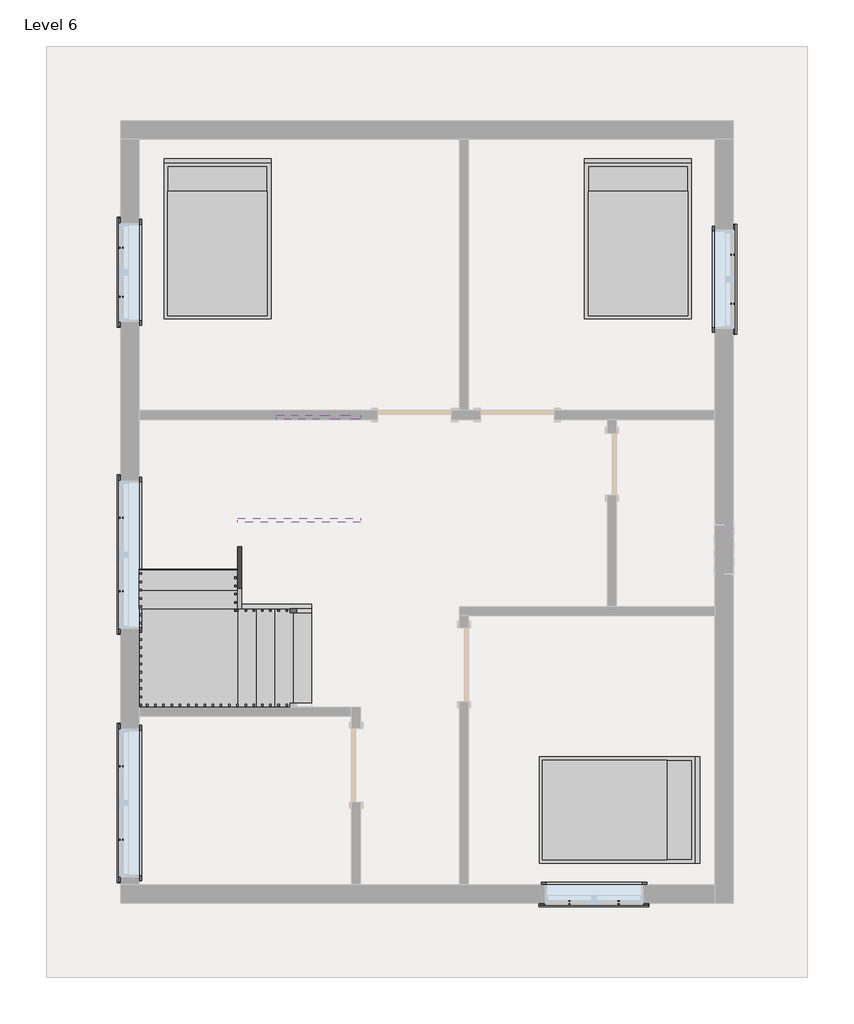
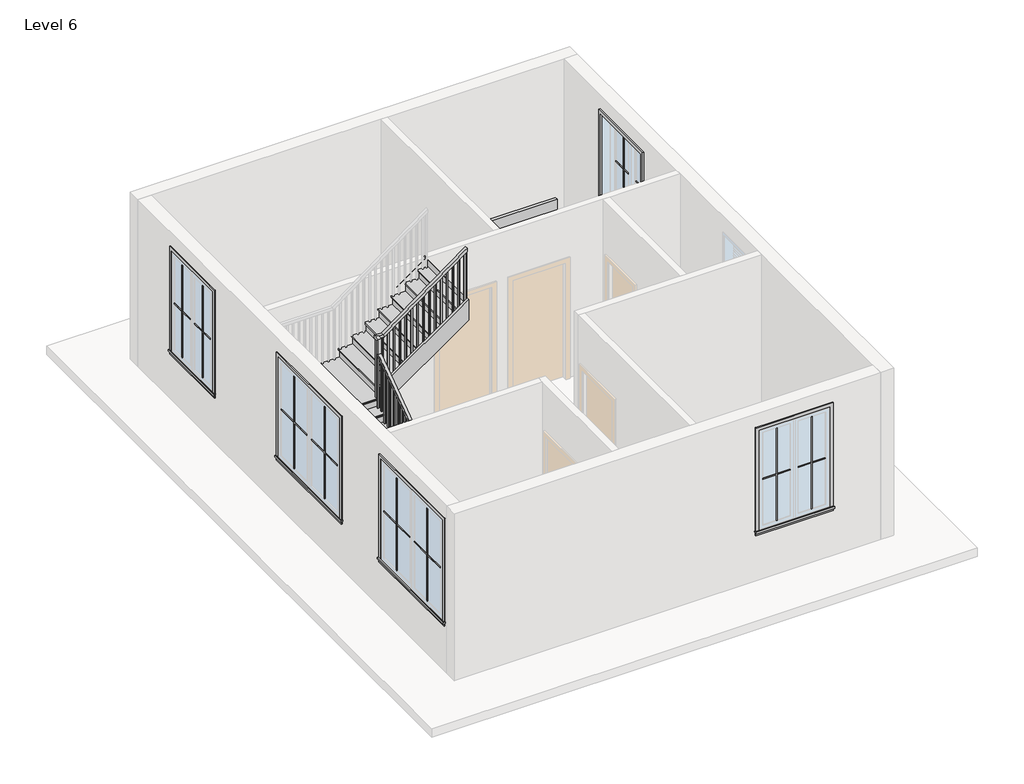
# One storey, part 2 of 2: 20 proxies, 5 members, 3 furniture elements, 1 railing, 1 stair flight.
"""IFC4 building model written with IfcOpenShell, lengths in millimetres."""

from ifc_helpers import new_model, si_unit, frame, origin, place, context, project, spatial, polyline, outline, extrude, faceted_brep, transform, mapped, element, save
from components import muntin_pattern_2x2_muntin_pattern_2x2_0a037076, muntin_pattern_2x2_muntin_pattern_2x2_e6f69628, muntin_pattern_2x2_muntin_pattern_2x2_2b4d9f72, muntin_pattern_2x2_muntin_pattern_2x2_ef995ed3, trim_window_exterior_flat_with_sill_b601e94a, trim_window_exterior_flat_with_sill_b7e4d11c, trim_window_interior_flat_picture_frame_bfefb25c, trim_window_interior_flat_picture_frame_936b8d2a, bed_17739_bed_17739_15c61121, stair_flight_8c9b7ea6

model = new_model("IFC4")

# Units and contexts
model_context = context("Model", 3, world=origin())
ifc_project = project(units=[si_unit("LENGTHUNIT", "METRE", prefix="MILLI")], contexts=[model_context])

# Site, building, storey
site = spatial("IfcSite", under=ifc_project)
building = spatial("IfcBuilding", under=site)
storey = spatial("IfcBuildingStorey", under=building, Name="Level 6", Elevation=15849.6)

# Proxies
placement = place(None, origin())
muntin_pattern_2x2_muntin_pattern_2x2_shape = muntin_pattern_2x2_muntin_pattern_2x2_0a037076(model_context)
element("IfcBuildingElementProxy", 1, Name="Muntin Pattern_2x2 : Muntin Pattern_2x2", ObjectType="Muntin Pattern_2x2 : Muntin Pattern_2x2", at=placement, inside=storey, context=model_context, shape_type="MappedRepresentation", body=[
    mapped(muntin_pattern_2x2_muntin_pattern_2x2_shape, transform((-5035.7855391, -4380.9248761, 16833.85), x_axis=(0.0, 1.0, 0.0), y_axis=(-1.0, 0.0, 0.0), z_axis=(0.0, 0.0, 1.0))),
])
element("IfcBuildingElementProxy", 2, Name="Muntin Pattern_2x2 : Muntin Pattern_2x2", ObjectType="Muntin Pattern_2x2 : Muntin Pattern_2x2", at=placement, inside=storey, context=model_context, shape_type="MappedRepresentation", body=[
    mapped(muntin_pattern_2x2_muntin_pattern_2x2_shape, transform((-5035.7855391, -1310.6998761, 16833.85), x_axis=(0.0, 1.0, 0.0), y_axis=(-1.0, 0.0, 0.0), z_axis=(0.0, 0.0, 1.0))),
])
muntin_pattern_2x2_muntin_pattern_2x2_2_shape = muntin_pattern_2x2_muntin_pattern_2x2_e6f69628(model_context)
element("IfcBuildingElementProxy", 3, Name="Muntin Pattern_2x2 : Muntin Pattern_2x2", ObjectType="Muntin Pattern_2x2 : Muntin Pattern_2x2", at=placement, inside=storey, context=model_context, shape_type="MappedRepresentation", body=[
    mapped(muntin_pattern_2x2_muntin_pattern_2x2_2_shape, transform((-5035.7855391, -3469.6998761, 16833.85), x_axis=(0.0, -1.0, 0.0), y_axis=(1.0, 0.0, 0.0), z_axis=(0.0, 0.0, 1.0))),
])
element("IfcBuildingElementProxy", 4, Name="Muntin Pattern_2x2 : Muntin Pattern_2x2", ObjectType="Muntin Pattern_2x2 : Muntin Pattern_2x2", at=placement, inside=storey, context=model_context, shape_type="MappedRepresentation", body=[
    mapped(muntin_pattern_2x2_muntin_pattern_2x2_2_shape, transform((-5035.7855391, -399.4748761, 16833.85), x_axis=(0.0, -1.0, 0.0), y_axis=(1.0, 0.0, 0.0), z_axis=(0.0, 0.0, 1.0))),
])
muntin_pattern_2x2_muntin_pattern_2x2_3_shape = muntin_pattern_2x2_muntin_pattern_2x2_2b4d9f72(model_context)
element("IfcBuildingElementProxy", 5, Name="Muntin Pattern_2x2 : Muntin Pattern_2x2", ObjectType="Muntin Pattern_2x2 : Muntin Pattern_2x2", at=placement, inside=storey, context=model_context, shape_type="MappedRepresentation", body=[
    mapped(muntin_pattern_2x2_muntin_pattern_2x2_3_shape, transform((1115.7769609, -5157.2123761, 16833.85), x_axis=(-1.0, 0.0, 0.0), y_axis=(0.0, -1.0, 0.0), z_axis=(0.0, 0.0, 1.0))),
])
element("IfcBuildingElementProxy", 6, Name="Muntin Pattern_2x2 : Muntin Pattern_2x2", ObjectType="Muntin Pattern_2x2 : Muntin Pattern_2x2", at=placement, inside=storey, context=model_context, shape_type="MappedRepresentation", body=[
    mapped(muntin_pattern_2x2_muntin_pattern_2x2_3_shape, transform((2527.0644609, 2851.7251239, 16833.85), x_axis=(0.0, -1.0, 0.0), y_axis=(1.0, 0.0, 0.0), z_axis=(0.0, 0.0, 1.0))),
])
element("IfcBuildingElementProxy", 7, Name="Muntin Pattern_2x2 : Muntin Pattern_2x2", ObjectType="Muntin Pattern_2x2 : Muntin Pattern_2x2", at=placement, inside=storey, context=model_context, shape_type="MappedRepresentation", body=[
    mapped(muntin_pattern_2x2_muntin_pattern_2x2_3_shape, transform((-5035.7855391, 2331.0251239, 16833.85), x_axis=(0.0, 1.0, 0.0), y_axis=(-1.0, 0.0, 0.0), z_axis=(0.0, 0.0, 1.0))),
])
muntin_pattern_2x2_muntin_pattern_2x2_4_shape = muntin_pattern_2x2_muntin_pattern_2x2_ef995ed3(model_context)
element("IfcBuildingElementProxy", 8, Name="Muntin Pattern_2x2 : Muntin Pattern_2x2", ObjectType="Muntin Pattern_2x2 : Muntin Pattern_2x2", at=placement, inside=storey, context=model_context, shape_type="MappedRepresentation", body=[
    mapped(muntin_pattern_2x2_muntin_pattern_2x2_4_shape, transform((509.3519609, -5157.2123761, 16833.85), x_axis=(1.0, 0.0, 0.0), y_axis=(0.0, 1.0, 0.0), z_axis=(0.0, 0.0, 1.0))),
])
element("IfcBuildingElementProxy", 9, Name="Muntin Pattern_2x2 : Muntin Pattern_2x2", ObjectType="Muntin Pattern_2x2 : Muntin Pattern_2x2", at=placement, inside=storey, context=model_context, shape_type="MappedRepresentation", body=[
    mapped(muntin_pattern_2x2_muntin_pattern_2x2_4_shape, transform((2527.0644609, 2245.3001239, 16833.85), x_axis=(0.0, 1.0, 0.0), y_axis=(-1.0, 0.0, 0.0), z_axis=(0.0, 0.0, 1.0))),
])
element("IfcBuildingElementProxy", 10, Name="Muntin Pattern_2x2 : Muntin Pattern_2x2", ObjectType="Muntin Pattern_2x2 : Muntin Pattern_2x2", at=placement, inside=storey, context=model_context, shape_type="MappedRepresentation", body=[
    mapped(muntin_pattern_2x2_muntin_pattern_2x2_4_shape, transform((-5035.7855391, 2937.4501239, 16833.85), x_axis=(0.0, -1.0, 0.0), y_axis=(1.0, 0.0, 0.0), z_axis=(0.0, 0.0, 1.0))),
])
trim_window_exterior_flat_with_sill_shape = trim_window_exterior_flat_with_sill_b601e94a(model_context)
element("IfcBuildingElementProxy", 11, Name="Trim-Window-Exterior-Flat : with Sill", ObjectType="Trim-Window-Exterior-Flat : with Sill", at=placement, inside=storey, context=model_context, shape_type="MappedRepresentation", body=[
    mapped(trim_window_exterior_flat_with_sill_shape, transform((-5045.3105391, -3925.3123761, 18592.8), x_axis=(0.0, -1.0, 0.0), y_axis=(0.0, 0.0, 1.0), z_axis=(-1.0, 0.0, 0.0))),
])
element("IfcBuildingElementProxy", 12, Name="Trim-Window-Exterior-Flat : with Sill", ObjectType="Trim-Window-Exterior-Flat : with Sill", at=placement, inside=storey, context=model_context, shape_type="MappedRepresentation", body=[
    mapped(trim_window_exterior_flat_with_sill_shape, transform((-5045.3105391, -855.0873761, 18592.8), x_axis=(0.0, -1.0, 0.0), y_axis=(0.0, 0.0, 1.0), z_axis=(-1.0, 0.0, 0.0))),
])
trim_window_exterior_flat_with_sill_2_shape = trim_window_exterior_flat_with_sill_b7e4d11c(model_context)
element("IfcBuildingElementProxy", 13, Name="Trim-Window-Exterior-Flat : with Sill", ObjectType="Trim-Window-Exterior-Flat : with Sill", at=placement, inside=storey, context=model_context, shape_type="MappedRepresentation", body=[
    mapped(trim_window_exterior_flat_with_sill_2_shape, transform((812.5644609, -5166.7373761, 18592.8), x_axis=(1.0, 0.0, 0.0), y_axis=(0.0, 0.0, 1.0), z_axis=(0.0, -1.0, 0.0))),
])
element("IfcBuildingElementProxy", 14, Name="Trim-Window-Exterior-Flat : with Sill", ObjectType="Trim-Window-Exterior-Flat : with Sill", at=placement, inside=storey, context=model_context, shape_type="MappedRepresentation", body=[
    mapped(trim_window_exterior_flat_with_sill_2_shape, transform((2536.5894609, 2548.5126239, 18592.8), x_axis=(0.0, 1.0, 0.0), y_axis=(0.0, 0.0, 1.0), z_axis=(1.0, 0.0, 0.0))),
])
element("IfcBuildingElementProxy", 15, Name="Trim-Window-Exterior-Flat : with Sill", ObjectType="Trim-Window-Exterior-Flat : with Sill", at=placement, inside=storey, context=model_context, shape_type="MappedRepresentation", body=[
    mapped(trim_window_exterior_flat_with_sill_2_shape, transform((-5045.3105391, 2634.2376239, 18592.8), x_axis=(0.0, -1.0, 0.0), y_axis=(0.0, 0.0, 1.0), z_axis=(-1.0, 0.0, 0.0))),
])
trim_window_interior_flat_picture_frame_shape = trim_window_interior_flat_picture_frame_bfefb25c(model_context)
element("IfcBuildingElementProxy", 16, Name="Trim-Window-Interior-Flat : Picture Frame", ObjectType="Trim-Window-Interior-Flat : Picture Frame", at=placement, inside=storey, context=model_context, shape_type="MappedRepresentation", body=[
    mapped(trim_window_interior_flat_picture_frame_shape, transform((-4816.7105391, -3925.3123761, 18592.8), x_axis=(0.0, 1.0, 0.0), y_axis=(0.0, 0.0, 1.0), z_axis=(1.0, 0.0, 0.0))),
])
element("IfcBuildingElementProxy", 17, Name="Trim-Window-Interior-Flat : Picture Frame", ObjectType="Trim-Window-Interior-Flat : Picture Frame", at=placement, inside=storey, context=model_context, shape_type="MappedRepresentation", body=[
    mapped(trim_window_interior_flat_picture_frame_shape, transform((-4816.7105391, -855.0873761, 18592.8), x_axis=(0.0, 1.0, 0.0), y_axis=(0.0, 0.0, 1.0), z_axis=(1.0, 0.0, 0.0))),
])
trim_window_interior_flat_picture_frame_2_shape = trim_window_interior_flat_picture_frame_936b8d2a(model_context)
element("IfcBuildingElementProxy", 18, Name="Trim-Window-Interior-Flat : Picture Frame", ObjectType="Trim-Window-Interior-Flat : Picture Frame", at=placement, inside=storey, context=model_context, shape_type="MappedRepresentation", body=[
    mapped(trim_window_interior_flat_picture_frame_2_shape, transform((812.5644609, -4938.1373761, 18592.8), x_axis=(-1.0, 0.0, 0.0), y_axis=(0.0, 0.0, 1.0), z_axis=(0.0, 1.0, 0.0))),
])
element("IfcBuildingElementProxy", 19, Name="Trim-Window-Interior-Flat : Picture Frame", ObjectType="Trim-Window-Interior-Flat : Picture Frame", at=placement, inside=storey, context=model_context, shape_type="MappedRepresentation", body=[
    mapped(trim_window_interior_flat_picture_frame_2_shape, transform((2307.9894609, 2548.5126239, 18592.8), x_axis=(0.0, -1.0, 0.0), y_axis=(0.0, 0.0, 1.0), z_axis=(-1.0, 0.0, 0.0))),
])
element("IfcBuildingElementProxy", 20, Name="Trim-Window-Interior-Flat : Picture Frame", ObjectType="Trim-Window-Interior-Flat : Picture Frame", at=placement, inside=storey, context=model_context, shape_type="MappedRepresentation", body=[
    mapped(trim_window_interior_flat_picture_frame_2_shape, transform((-4816.7105391, 2634.2376239, 18592.8), x_axis=(0.0, 1.0, 0.0), y_axis=(0.0, 0.0, 1.0), z_axis=(1.0, 0.0, 0.0))),
])

# Furniture
bed_17739_bed_17739_shape = bed_17739_bed_17739_15c61121(model_context)
element("IfcFurniture", 21, ObjectType="Bed_17739 : Bed_17739", at=placement, inside=storey, context=model_context, shape_type="MappedRepresentation", body=[
    mapped(bed_17739_bed_17739_shape, transform((-3845.1605391, 3024.7626239, 15849.6), x_axis=(1.0, 0.0, 0.0), y_axis=(0.0, 1.0, 0.0), z_axis=(0.0, 0.0, 1.0))),
])
element("IfcFurniture", 22, ObjectType="Bed_17739 : Bed_17739", at=placement, inside=storey, context=model_context, shape_type="MappedRepresentation", body=[
    mapped(bed_17739_bed_17739_shape, transform((1355.4894609, 3024.7626239, 15849.6), x_axis=(1.0, 0.0, 0.0), y_axis=(0.0, 1.0, 0.0), z_axis=(0.0, 0.0, 1.0))),
])
element("IfcFurniture", 23, ObjectType="Bed_17739 : Bed_17739", at=placement, inside=storey, context=model_context, shape_type="MappedRepresentation", body=[
    mapped(bed_17739_bed_17739_shape, transform((1101.4894609, -4011.0373761, 15849.6), x_axis=(0.0, -1.0, 0.0), y_axis=(1.0, 0.0, 0.0), z_axis=(0.0, 0.0, 1.0))),
])

# Members
element("IfcMember", 24, ObjectType="Stringer - 2\" Width", at=placement, inside=storey, context=model_context, shape_type="SweptSolid", body=[
    extrude(outline(polyline([(15849.6, -2683.1105391), (16000.1087903, -2683.1105391), (16000.1087903, -3112.2707489), (15849.6, -2897.7957228), (15849.6, -2683.1105391)])), frame((0.0, -2791.8373761, 0.0), z_axis=(0.0, 1.0, 0.0), x_axis=(0.0, 0.0, 1.0)), (0.0, 0.0, 1.0), 50.8),
])
element("IfcMember", 25, ObjectType="Stringer - 2\" Width", at=placement, inside=storey, context=model_context, shape_type="SweptSolid", body=[
    extrude(outline(polyline([(18177.0856495, -2580.7583047), (18533.0489938, -2073.5105391), (18905.4117181, -2073.5105391), (18177.0856495, -3111.3751869), (18177.0856495, -2580.7583047)])), frame((0.0, 814.9626239, 0.0), z_axis=(0.0, 1.0, 0.0), x_axis=(0.0, 0.0, 1.0)), (0.0, 0.0, 1.0), 50.8),
])
element("IfcMember", 26, ObjectType="Stringer - 2\" Width", at=placement, inside=storey, context=model_context, shape_type="SweptSolid", body=[
    extrude(outline(polyline([(15849.6, -2683.1105391), (16071.306455, -2683.1105391), (16677.3415427, -3546.7105391), (16304.9788184, -3546.7105391), (15849.6, -2897.7957228), (15849.6, -2683.1105391)])), frame((0.0, -1521.8373761, 0.0), z_axis=(0.0, 1.0, 0.0), x_axis=(0.0, 0.0, 1.0)), (0.0, 0.0, 1.0), 50.8),
])
element("IfcMember", 27, ObjectType="Stringer - 2\" Width", at=placement, inside=storey, context=model_context, shape_type="SweptSolid", body=[
    extrude(outline(polyline([(-1521.8373761, 16499.9564629), (-1521.8373761, 16875.1327137), (-455.0373761, 17640.7786467), (-455.0373761, 17265.6023959), (-1521.8373761, 16499.9564629)])), frame((-3597.5105391, 0.0, 0.0), z_axis=(1.0, 0.0, 0.0), x_axis=(0.0, 1.0, 0.0)), (0.0, 0.0, 1.0), 50.8),
])
element("IfcMember", 28, ObjectType="Stringer - 2\" Width", at=placement, inside=storey, context=model_context, shape_type="SweptSolid", body=[
    extrude(outline(polyline([(17835.9380339, -3597.5105391), (17463.5753096, -3597.5105391), (18533.0489938, -2073.5105391), (18905.4117181, -2073.5105391), (17835.9380339, -3597.5105391)])), frame((0.0, -455.0373761, 0.0), z_axis=(0.0, 1.0, 0.0), x_axis=(0.0, 0.0, 1.0)), (0.0, 0.0, 1.0), 50.8),
])

# Railing
element("IfcRailing", 29, ObjectType="Handrail - Rectangular", at=placement, inside=storey, context=model_context, shape_type="SolidModel", body=[
    faceted_brep([(-2683.1105391, -1572.6373761, 16924.4210526), (-2683.1105391, -1572.6373761, 16862.3605986), (-2683.1105391, -1521.8373761, 16862.3605986), (-2683.1105391, -1521.8373761, 16924.4210526), (-3521.3105391, -1572.6373761, 17512.6315789), (-3572.1105391, -1572.6373761, 17486.2202477), (-3572.1105391, -1521.8373761, 17486.2202477), (-3521.3105391, -1521.8373761, 17512.6315789), (-3521.3105391, -1572.6373761, 17781.215311), (-3572.1105391, -1572.6373761, 17730.415311), (-3572.1105391, -1521.8373761, 17730.415311), (-3521.3105391, -1521.8373761, 17781.215311), (-3648.3105391, -1572.6373761, 17781.215311), (-3648.3105391, -1572.6373761, 17730.415311), (-3597.5105391, -1521.8373761, 17730.415311), (-3597.5105391, -1521.8373761, 17781.215311), (-3648.3105391, -1445.6373761, 17781.215311), (-3648.3105391, -1429.2944467, 17730.415311), (-3597.5105391, -1429.2944467, 17730.415311), (-3597.5105391, -1445.6373761, 17781.215311), (-3648.3105391, -480.4373761, 18473.9425837), (-3648.3105391, -429.6373761, 18447.8725387), (-3597.5105391, -429.6373761, 18447.8725387), (-3597.5105391, -480.4373761, 18473.9425837), (-3648.3105391, -480.4373761, 18745.2), (-3648.3105391, -429.6373761, 18694.4), (-3597.5105391, -429.6373761, 18694.4), (-3597.5105391, -480.4373761, 18745.2), (-3648.3105391, -353.4373761, 18745.2), (-3648.3105391, -353.4373761, 18694.4), (-3597.5105391, -404.2373761, 18694.4), (-3597.5105391, -404.2373761, 18745.2), (-3521.3105391, -353.4373761, 18745.2), (-3504.6160355, -353.4373761, 18694.4), (-3504.6160355, -404.2373761, 18694.4), (-3521.3105391, -404.2373761, 18745.2), (-2073.5105391, -353.4373761, 19812.0), (-2073.5105391, -404.2373761, 19812.0), (-2073.5105391, -404.2373761, 19748.8987868), (-2073.5105391, -353.4373761, 19748.8987868)], [[[0, 1, 2, 3]], [[1, 0, 4, 5]], [[2, 1, 5, 6]], [[3, 2, 6, 7]], [[0, 3, 7, 4]], [[5, 4, 8, 9]], [[6, 5, 9, 10]], [[7, 6, 10, 11]], [[4, 7, 11, 8]], [[9, 8, 12, 13]], [[10, 9, 13, 14]], [[11, 10, 14, 15]], [[8, 11, 15, 12]], [[13, 12, 16, 17]], [[14, 13, 17, 18]], [[15, 14, 18, 19]], [[12, 15, 19, 16]], [[17, 16, 20, 21]], [[18, 17, 21, 22]], [[19, 18, 22, 23]], [[16, 19, 23, 20]], [[21, 20, 24, 25]], [[22, 21, 25, 26]], [[23, 22, 26, 27]], [[20, 23, 27, 24]], [[25, 24, 28, 29]], [[26, 25, 29, 30]], [[27, 26, 30, 31]], [[24, 27, 31, 28]], [[29, 28, 32, 33]], [[30, 29, 33, 34]], [[31, 30, 34, 35]], [[28, 31, 35, 32]], [[36, 37, 38, 39]], [[33, 32, 36, 39]], [[34, 33, 39, 38]], [[35, 34, 38, 37]], [[32, 35, 37, 36]]]),
    extrude(outline(polyline([(19737.2014184, -2089.3855391), (19723.1645763, -2108.4355391), (18737.1789474, -2108.4355391), (18737.1789474, -2089.3855391), (19737.2014184, -2089.3855391)])), frame((0.0, -388.3623761, 0.0), z_axis=(0.0, 1.0, 0.0), x_axis=(0.0, 0.0, 1.0)), (0.0, 0.0, 1.0), 19.05),
    extrude(outline(polyline([(19662.3382605, -2190.9855391), (19648.3014184, -2210.0355391), (18737.1789474, -2210.0355391), (18737.1789474, -2190.9855391), (19662.3382605, -2190.9855391)])), frame((0.0, -388.3623761, 0.0), z_axis=(0.0, 1.0, 0.0), x_axis=(0.0, 0.0, 1.0)), (0.0, 0.0, 1.0), 19.05),
    extrude(outline(polyline([(19587.4751026, -2292.5855391), (19573.4382605, -2311.6355391), (18576.7578947, -2311.6355391), (18576.7578947, -2292.5855391), (19587.4751026, -2292.5855391)])), frame((0.0, -388.3623761, 0.0), z_axis=(0.0, 1.0, 0.0), x_axis=(0.0, 0.0, 1.0)), (0.0, 0.0, 1.0), 19.05),
    extrude(outline(polyline([(19512.6119447, -2394.1855391), (19498.5751026, -2413.2355391), (18576.7578947, -2413.2355391), (18576.7578947, -2394.1855391), (19512.6119447, -2394.1855391)])), frame((0.0, -388.3623761, 0.0), z_axis=(0.0, 1.0, 0.0), x_axis=(0.0, 0.0, 1.0)), (0.0, 0.0, 1.0), 19.05),
    extrude(outline(polyline([(19437.7487868, -2495.7855391), (19423.7119447, -2514.8355391), (18416.3368421, -2514.8355391), (18416.3368421, -2495.7855391), (19437.7487868, -2495.7855391)])), frame((0.0, -388.3623761, 0.0), z_axis=(0.0, 1.0, 0.0), x_axis=(0.0, 0.0, 1.0)), (0.0, 0.0, 1.0), 19.05),
    extrude(outline(polyline([(19362.8856289, -2597.3855391), (19348.8487868, -2616.4355391), (18416.3368421, -2616.4355391), (18416.3368421, -2597.3855391), (19362.8856289, -2597.3855391)])), frame((0.0, -388.3623761, 0.0), z_axis=(0.0, 1.0, 0.0), x_axis=(0.0, 0.0, 1.0)), (0.0, 0.0, 1.0), 19.05),
    extrude(outline(polyline([(19288.022471, -2698.9855391), (19273.9856289, -2718.0355391), (18255.9157895, -2718.0355391), (18255.9157895, -2698.9855391), (19288.022471, -2698.9855391)])), frame((0.0, -388.3623761, 0.0), z_axis=(0.0, 1.0, 0.0), x_axis=(0.0, 0.0, 1.0)), (0.0, 0.0, 1.0), 19.05),
    extrude(outline(polyline([(19213.1593132, -2800.5855391), (19199.122471, -2819.6355391), (18255.9157895, -2819.6355391), (18255.9157895, -2800.5855391), (19213.1593132, -2800.5855391)])), frame((0.0, -388.3623761, 0.0), z_axis=(0.0, 1.0, 0.0), x_axis=(0.0, 0.0, 1.0)), (0.0, 0.0, 1.0), 19.05),
    extrude(outline(polyline([(19138.2961553, -2902.1855391), (19124.2593132, -2921.2355391), (18255.9157895, -2921.2355391), (18255.9157895, -2902.1855391), (19138.2961553, -2902.1855391)])), frame((0.0, -388.3623761, 0.0), z_axis=(0.0, 1.0, 0.0), x_axis=(0.0, 0.0, 1.0)), (0.0, 0.0, 1.0), 19.05),
    extrude(outline(polyline([(19063.4329974, -3003.7855391), (19049.3961553, -3022.8355391), (18095.4947368, -3022.8355391), (18095.4947368, -3003.7855391), (19063.4329974, -3003.7855391)])), frame((0.0, -388.3623761, 0.0), z_axis=(0.0, 1.0, 0.0), x_axis=(0.0, 0.0, 1.0)), (0.0, 0.0, 1.0), 19.05),
    extrude(outline(polyline([(18988.5698395, -3105.3855391), (18974.5329974, -3124.4355391), (18095.4947368, -3124.4355391), (18095.4947368, -3105.3855391), (18988.5698395, -3105.3855391)])), frame((0.0, -388.3623761, 0.0), z_axis=(0.0, 1.0, 0.0), x_axis=(0.0, 0.0, 1.0)), (0.0, 0.0, 1.0), 19.05),
    extrude(outline(polyline([(18913.7066816, -3206.9855391), (18899.6698395, -3226.0355391), (17935.0736842, -3226.0355391), (17935.0736842, -3206.9855391), (18913.7066816, -3206.9855391)])), frame((0.0, -388.3623761, 0.0), z_axis=(0.0, 1.0, 0.0), x_axis=(0.0, 0.0, 1.0)), (0.0, 0.0, 1.0), 19.05),
    extrude(outline(polyline([(18838.8435237, -3308.5855391), (18824.8066816, -3327.6355391), (17935.0736842, -3327.6355391), (17935.0736842, -3308.5855391), (18838.8435237, -3308.5855391)])), frame((0.0, -388.3623761, 0.0), z_axis=(0.0, 1.0, 0.0), x_axis=(0.0, 0.0, 1.0)), (0.0, 0.0, 1.0), 19.05),
    extrude(outline(polyline([(18763.9803658, -3410.1855391), (18749.9435237, -3429.2355391), (17774.6526316, -3429.2355391), (17774.6526316, -3410.1855391), (18763.9803658, -3410.1855391)])), frame((0.0, -388.3623761, 0.0), z_axis=(0.0, 1.0, 0.0), x_axis=(0.0, 0.0, 1.0)), (0.0, 0.0, 1.0), 19.05),
    extrude(outline(polyline([(18689.1172079, -3511.7855391), (18675.0803658, -3530.8355391), (17774.6526316, -3530.8355391), (17774.6526316, -3511.7855391), (18689.1172079, -3511.7855391)])), frame((0.0, -388.3623761, 0.0), z_axis=(0.0, 1.0, 0.0), x_axis=(0.0, 0.0, 1.0)), (0.0, 0.0, 1.0), 19.05),
    extrude(outline(polyline([(-3613.3855391, -439.1623761), (-3632.4355391, -439.1623761), (-3632.4355391, -420.1123761), (-3613.3855391, -420.1123761), (-3613.3855391, -439.1623761)])), frame((0.0, 0.0, 17453.8105263), z_axis=(0.0, 0.0, 1.0), x_axis=(1.0, 0.0, 0.0)), (0.0, 0.0, 1.0), 1240.5894737),
    extrude(outline(polyline([(-540.7623761, 18368.1177541), (-521.7123761, 18381.7900029), (-521.7123761, 17453.8105263), (-540.7623761, 17453.8105263), (-540.7623761, 18368.1177541)])), frame((-3632.4355391, 0.0, 0.0), z_axis=(1.0, 0.0, 0.0), x_axis=(0.0, 1.0, 0.0)), (0.0, 0.0, 1.0), 19.05),
    extrude(outline(polyline([(-642.3623761, 18295.1990938), (-623.3123761, 18308.8713426), (-623.3123761, 17293.3894737), (-642.3623761, 17293.3894737), (-642.3623761, 18295.1990938)])), frame((-3632.4355391, 0.0, 0.0), z_axis=(1.0, 0.0, 0.0), x_axis=(0.0, 1.0, 0.0)), (0.0, 0.0, 1.0), 19.05),
    extrude(outline(polyline([(-743.9623761, 18222.2804335), (-724.9123761, 18235.9526823), (-724.9123761, 17293.3894737), (-743.9623761, 17293.3894737), (-743.9623761, 18222.2804335)])), frame((-3632.4355391, 0.0, 0.0), z_axis=(1.0, 0.0, 0.0), x_axis=(0.0, 1.0, 0.0)), (0.0, 0.0, 1.0), 19.05),
    extrude(outline(polyline([(-845.5623761, 18149.3617732), (-826.5123761, 18163.034022), (-826.5123761, 17293.3894737), (-845.5623761, 17293.3894737), (-845.5623761, 18149.3617732)])), frame((-3632.4355391, 0.0, 0.0), z_axis=(1.0, 0.0, 0.0), x_axis=(0.0, 1.0, 0.0)), (0.0, 0.0, 1.0), 19.05),
    extrude(outline(polyline([(-947.1623761, 18076.4431129), (-928.1123761, 18090.1153617), (-928.1123761, 17132.9684211), (-947.1623761, 17132.9684211), (-947.1623761, 18076.4431129)])), frame((-3632.4355391, 0.0, 0.0), z_axis=(1.0, 0.0, 0.0), x_axis=(0.0, 1.0, 0.0)), (0.0, 0.0, 1.0), 19.05),
    extrude(outline(polyline([(-1048.7623761, 18003.5244526), (-1029.7123761, 18017.1967014), (-1029.7123761, 17132.9684211), (-1048.7623761, 17132.9684211), (-1048.7623761, 18003.5244526)])), frame((-3632.4355391, 0.0, 0.0), z_axis=(1.0, 0.0, 0.0), x_axis=(0.0, 1.0, 0.0)), (0.0, 0.0, 1.0), 19.05),
    extrude(outline(polyline([(-1150.3623761, 17930.6057923), (-1131.3123761, 17944.2780411), (-1131.3123761, 16972.5473684), (-1150.3623761, 16972.5473684), (-1150.3623761, 17930.6057923)])), frame((-3632.4355391, 0.0, 0.0), z_axis=(1.0, 0.0, 0.0), x_axis=(0.0, 1.0, 0.0)), (0.0, 0.0, 1.0), 19.05),
    extrude(outline(polyline([(-1251.9623761, 17857.687132), (-1232.9123761, 17871.3593808), (-1232.9123761, 16972.5473684), (-1251.9623761, 16972.5473684), (-1251.9623761, 17857.687132)])), frame((-3632.4355391, 0.0, 0.0), z_axis=(1.0, 0.0, 0.0), x_axis=(0.0, 1.0, 0.0)), (0.0, 0.0, 1.0), 19.05),
    extrude(outline(polyline([(-1353.5623761, 17784.7684718), (-1334.5123761, 17798.4407206), (-1334.5123761, 16812.1263158), (-1353.5623761, 16812.1263158), (-1353.5623761, 17784.7684718)])), frame((-3632.4355391, 0.0, 0.0), z_axis=(1.0, 0.0, 0.0), x_axis=(0.0, 1.0, 0.0)), (0.0, 0.0, 1.0), 19.05),
    extrude(outline(polyline([(-1455.1623761, 17711.8498115), (-1436.1123761, 17725.5220603), (-1436.1123761, 16812.1263158), (-1455.1623761, 16812.1263158), (-1455.1623761, 17711.8498115)])), frame((-3632.4355391, 0.0, 0.0), z_axis=(1.0, 0.0, 0.0), x_axis=(0.0, 1.0, 0.0)), (0.0, 0.0, 1.0), 19.05),
    extrude(outline(polyline([(-3587.9855391, -1537.7123761), (-3587.9855391, -1556.7623761), (-3607.0355391, -1556.7623761), (-3607.0355391, -1537.7123761), (-3587.9855391, -1537.7123761)])), frame((0.0, 0.0, 16651.7052632), z_axis=(0.0, 0.0, 1.0), x_axis=(1.0, 0.0, 0.0)), (0.0, 0.0, 1.0), 1078.7100478),
    extrude(outline(polyline([(17426.062353, -3486.3855391), (17439.430774, -3505.4355391), (16491.2842105, -3505.4355391), (16491.2842105, -3486.3855391), (17426.062353, -3486.3855391)])), frame((0.0, -1556.7623761, 0.0), z_axis=(0.0, 1.0, 0.0), x_axis=(0.0, 0.0, 1.0)), (0.0, 0.0, 1.0), 19.05),
    extrude(outline(polyline([(17354.7641074, -3384.7855391), (17368.1325284, -3403.8355391), (16491.2842105, -3403.8355391), (16491.2842105, -3384.7855391), (17354.7641074, -3384.7855391)])), frame((0.0, -1556.7623761, 0.0), z_axis=(0.0, 1.0, 0.0), x_axis=(0.0, 0.0, 1.0)), (0.0, 0.0, 1.0), 19.05),
    extrude(outline(polyline([(17283.4658617, -3283.1855391), (17296.8342828, -3302.2355391), (16330.8631579, -3302.2355391), (16330.8631579, -3283.1855391), (17283.4658617, -3283.1855391)])), frame((0.0, -1556.7623761, 0.0), z_axis=(0.0, 1.0, 0.0), x_axis=(0.0, 0.0, 1.0)), (0.0, 0.0, 1.0), 19.05),
    extrude(outline(polyline([(17212.1676161, -3181.5855391), (17225.5360372, -3200.6355391), (16330.8631579, -3200.6355391), (16330.8631579, -3181.5855391), (17212.1676161, -3181.5855391)])), frame((0.0, -1556.7623761, 0.0), z_axis=(0.0, 1.0, 0.0), x_axis=(0.0, 0.0, 1.0)), (0.0, 0.0, 1.0), 19.05),
    extrude(outline(polyline([(17140.8693705, -3079.9855391), (17154.2377916, -3099.0355391), (16170.4421053, -3099.0355391), (16170.4421053, -3079.9855391), (17140.8693705, -3079.9855391)])), frame((0.0, -1556.7623761, 0.0), z_axis=(0.0, 1.0, 0.0), x_axis=(0.0, 0.0, 1.0)), (0.0, 0.0, 1.0), 19.05),
    extrude(outline(polyline([(17069.5711249, -2978.3855391), (17082.9395459, -2997.4355391), (16170.4421053, -2997.4355391), (16170.4421053, -2978.3855391), (17069.5711249, -2978.3855391)])), frame((0.0, -1556.7623761, 0.0), z_axis=(0.0, 1.0, 0.0), x_axis=(0.0, 0.0, 1.0)), (0.0, 0.0, 1.0), 19.05),
    extrude(outline(polyline([(16998.2728793, -2876.7855391), (17011.6413003, -2895.8355391), (16010.0210526, -2895.8355391), (16010.0210526, -2876.7855391), (16998.2728793, -2876.7855391)])), frame((0.0, -1556.7623761, 0.0), z_axis=(0.0, 1.0, 0.0), x_axis=(0.0, 0.0, 1.0)), (0.0, 0.0, 1.0), 19.05),
    extrude(outline(polyline([(16926.9746337, -2775.1855391), (16940.3430547, -2794.2355391), (16010.0210526, -2794.2355391), (16010.0210526, -2775.1855391), (16926.9746337, -2775.1855391)])), frame((0.0, -1556.7623761, 0.0), z_axis=(0.0, 1.0, 0.0), x_axis=(0.0, 0.0, 1.0)), (0.0, 0.0, 1.0), 19.05),
    extrude(outline(polyline([(-3613.3855391, -388.3623761), (-3632.4355391, -388.3623761), (-3632.4355391, -369.3123761), (-3613.3855391, -369.3123761), (-3613.3855391, -388.3623761)])), frame((0.0, 0.0, 17614.2315789), z_axis=(0.0, 0.0, 1.0), x_axis=(1.0, 0.0, 0.0)), (0.0, 0.0, 1.0), 1080.1684211),
    extrude(outline(polyline([(-3613.3855391, -1537.7123761), (-3613.3855391, -1556.7623761), (-3632.4355391, -1556.7623761), (-3632.4355391, -1537.7123761), (-3613.3855391, -1537.7123761)])), frame((0.0, 0.0, 16651.7052632), z_axis=(0.0, 0.0, 1.0), x_axis=(1.0, 0.0, 0.0)), (0.0, 0.0, 1.0), 1078.7100478),
    extrude(outline(polyline([(19748.8987868, -2073.5105391), (19734.8619447, -2092.5605391), (18737.1789474, -2092.5605391), (18737.1789474, -2073.5105391), (19748.8987868, -2073.5105391)])), frame((0.0, -388.3623761, 0.0), z_axis=(0.0, 1.0, 0.0), x_axis=(0.0, 0.0, 1.0)), (0.0, 0.0, 1.0), 19.05),
    extrude(outline(polyline([(16862.3605986, -2683.1105391), (16875.7290196, -2702.1605391), (16010.0210526, -2702.1605391), (16010.0210526, -2683.1105391), (16862.3605986, -2683.1105391)])), frame((0.0, -1556.7623761, 0.0), z_axis=(0.0, 1.0, 0.0), x_axis=(0.0, 0.0, 1.0)), (0.0, 0.0, 1.0), 19.05),
])

# Stair flight
stair_flight_shape = stair_flight_8c9b7ea6(model_context)
element("IfcStairFlight", 30, ObjectType="2\" Tread 1\" Nosing 1/4\" Riser", at=placement, inside=storey, context=model_context, shape_type="MappedRepresentation", body=[
    mapped(stair_flight_shape, transform((0.0, 0.0, 0.0), x_axis=(1.0, 0.0, 0.0), y_axis=(0.0, 1.0, 0.0), z_axis=(0.0, 0.0, 1.0))),
])

save(model, "model.ifc")

# Revit data of these elements
# Type "Muntin Pattern_2x2 : Muntin Pattern_2x2"
#   Width [instance default] = 4' - 0"
#   Thickness = 0' - 0 1/2"
#   Height [instance default] = 4' - 0"
#   Distance = 0' - 0 3/4"
#   Interior Material [instance default] = none
#   Exterior Material [instance default] = none
#   Default Elevation = 0
# Type "Trim-Window-Exterior-Flat : with Sill"
#   Trim Width = 0' - 2 1/4"
#   Trim Thickness_Picture Frame = 0' - 1 1/4"
#   Trim Thickness_with Sill = 0' - 0 3/4"
#   Sill Thickness = 0' - 1 1/4"
#   Opening Width [instance default] = 2' - 0"
#   Opening Height [instance default] = 3' - 0"
#   Default Elevation = 4' - 0"
#   Sill = yes
#   Picture Frame = no
#   Trim Material [instance default] = none
# Type "Trim-Window-Interior-Flat : Picture Frame"
#   Trim Thickness_Picture Frame = 0' - 1 1/4"
#   Trim Width = 0' - 2 1/4"
#   Trim Thickness_with Sill = 0' - 0 3/4"
#   Sill Thickness = 0' - 1 1/4"
#   Opening Width [instance default] = 2' - 0"
#   Opening Height [instance default] = 3' - 0"
#   Default Elevation = 4' - 0"
#   Sill = no
#   Picture Frame = yes
#   Trim Material [instance default] = none
# Type "Bed_17739 : Bed_17739"
#   Default Elevation = 0
# Type "Handrail - Rectangular"
#   Assembly Code = "C2010400"
#   built-in parameter 1008612 = 0.0416667 (stored number, unit not read)
#   built-in parameter 1008611 = 0.0416667 (stored number, unit not read)
#   built-in parameter 1008609 = 0.333333 (stored number, unit not read)
#   built-in parameter 1008604 = 0.166667 (stored number, unit not read)
#   built-in parameter 1008603 = 0.166667 (stored number, unit not read)
#   Railing Height = 3' - 0"
#   built-in parameter 1008630 = 2
#   built-in parameter 1008610 = 2
#   built-in parameter 1008618 = Baluster - Square : 3/4"
# Elements 1, 2, 3, 4 (IfcBuildingElementProxy, "Muntin Pattern_2x2 : Muntin Pattern_2x2")
#   Width = 2' - 6 5/8"
#   Height = 5' - 6 1/2"
#   Interior Material = Wood - Stained
#   Exterior Material = Clad - White
#   Phase Created = New Construction
#   Materials on its faces: "Clad - White", "Wood - Stained"
# Elements 5, 6, 7, 8, 9, 10 (IfcBuildingElementProxy, "Muntin Pattern_2x2 : Muntin Pattern_2x2")
#   Width = 1' - 6 5/8"
#   Height = 5' - 6 1/2"
#   Interior Material = Wood - Stained
#   Exterior Material = Clad - White
#   Phase Created = New Construction
#   Materials on its faces: "Clad - White", "Wood - Stained"
# Elements 11, 12 (IfcBuildingElementProxy, "Trim-Window-Exterior-Flat : with Sill")
#   Opening Width = 6' - 0"
#   Opening Height = 6' - 0"
#   Trim Material = Clad - White
#   Phase Created = New Construction
#   Materials on its faces: "Clad - White"
# Elements 13, 14, 15 (IfcBuildingElementProxy, "Trim-Window-Exterior-Flat : with Sill")
#   Opening Width = 4' - 0"
#   Opening Height = 6' - 0"
#   Trim Material = Clad - White
#   Phase Created = New Construction
#   Materials on its faces: "Clad - White"
# Elements 16, 17 (IfcBuildingElementProxy, "Trim-Window-Interior-Flat : Picture Frame")
#   Opening Width = 6' - 0"
#   Opening Height = 6' - 0"
#   Trim Material = Wood - Stained
#   Phase Created = New Construction
#   Materials on its faces: "Wood - Stained"
# Elements 18, 19, 20 (IfcBuildingElementProxy, "Trim-Window-Interior-Flat : Picture Frame")
#   Opening Width = 4' - 0"
#   Opening Height = 6' - 0"
#   Trim Material = Wood - Stained
#   Phase Created = New Construction
#   Materials on its faces: "Wood - Stained"
# Elements 21, 22, 23 (IfcFurniture, "Bed_17739 : Bed_17739")
#   Phase Created = New Construction
#   Materials on its faces: "legs", "sheets", "bed frame", "Blanket"
# Elements 24, 25, 26, 27, 28 (IfcMember, "Stringer - 2\" Width")
#   Phase Created = New Construction
# Element 29 (IfcRailing, "Handrail - Rectangular")
#   Phase Created = New Construction
# Element 30 (IfcStairFlight, "2\" Tread 1\" Nosing 1/4\" Riser")
#   Phase Created = New Construction
# Materials
#   "Clad - White": class "Wood", colour RGB 242 242 238, transparency 0, Cost = 0
#   "Wood - Stained": class "Wood", colour RGB 224 178 126, transparency 0, Cost = 0
#   "legs": colour RGB 90 73 37, transparency 0, Cost = 0
#   "sheets": colour RGB 200 195 176, transparency 0, Cost = 0
#   "bed frame": colour RGB 90 73 37, transparency 0, Cost = 0
#   "Blanket": class "System", colour RGB 59 0 1, transparency 0, Cost = 0
